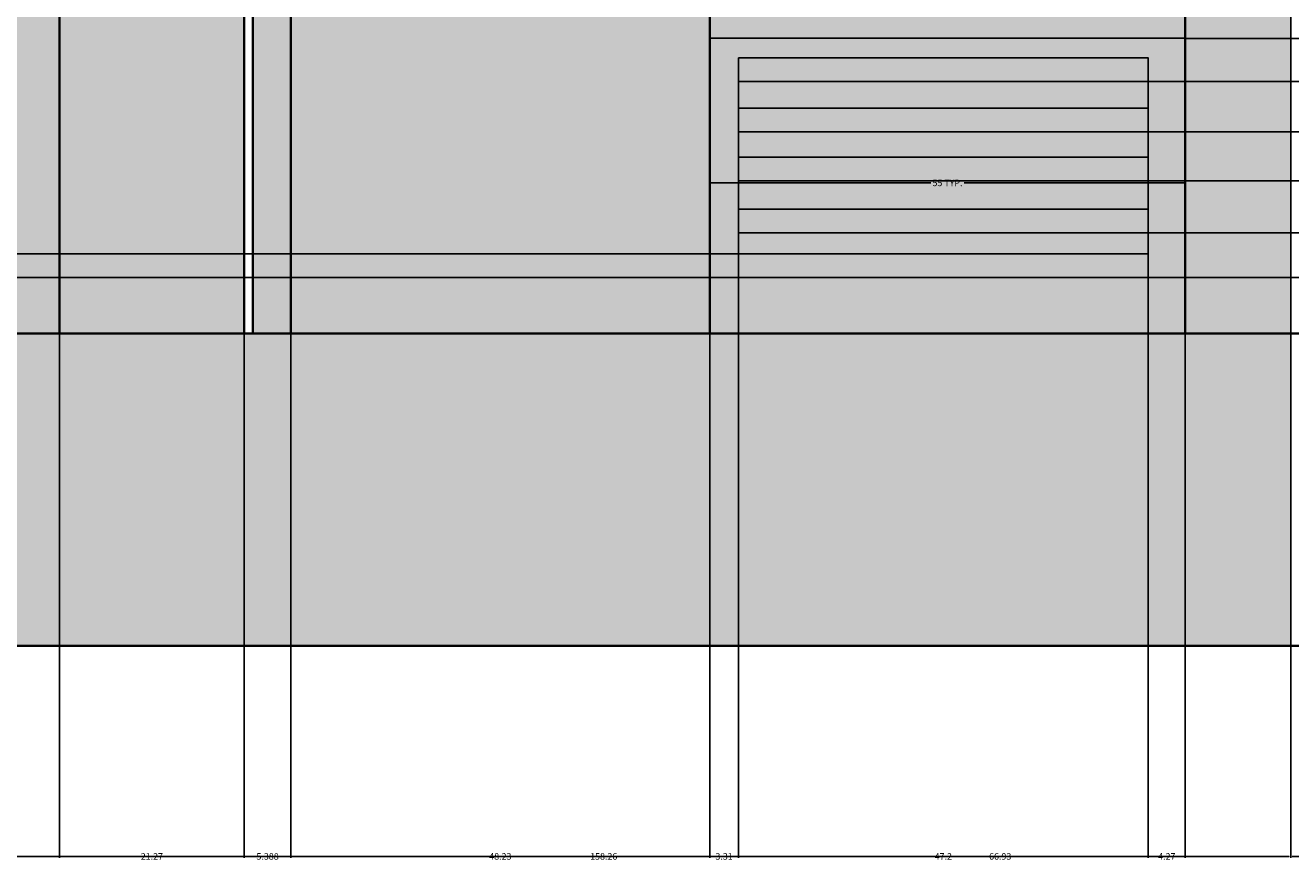
# Model space of a CAD drawing. Units: inches. Extents: x 62 to 566, y 66 to 528.
# Tile 3 of 20: x 138 to 284, y 66 to 162. Entities that reach past the tile are written whole.
import ezdxf

# ---------------------------------------------------------------- set-up
doc = ezdxf.new("R2010")
doc.units = ezdxf.units.IN
doc.header["$MEASUREMENT"] = 0
for name, color, linetype, lineweight in [('A-ANNO-DIMS', 2, 'Continuous', 18), ('A-ELEV', 7, 'Continuous', 35), ('A-GLAZ', 3, 'Continuous', 25), ('A-WALL-PATT', 8, 'Continuous', 13)]:
    doc.layers.add(name, color=color, linetype=linetype, lineweight=lineweight)
doc.styles.get("Standard").update_dxf_attribs({"font": 'arial.ttf'})
doc.dimstyles.get("Standard").update_dxf_attribs({"dimtxt": 0.75, "dimasz": 0.18, "dimexe": 0.18, "dimexo": 0.0625, "dimgap": 0.09, "dimtad": 0, "dimtih": 1, "dimtoh": 1, "dimdec": 4, "dimzin": 0, "dimdsep": 46, "dimlunit": 4, "dimtxsty": 'Standard', "dimcen": 0.09, "dimadec": 0, "dimazin": 0, "dimtfac": 1, "dimtdec": 4, "dimtofl": 0, "dimtmove": 0, "dimatfit": 3, "dimfxl": 1, "dimtolj": 1, "dimtzin": 0, "dimarcsym": 0})

# ---------------------------------------------------------------- blocks, each defined once
blk = doc.blocks.new('WIN-FRENCH-GRID')
for p, q in [((26.39, 108.06), (26.39, 83.9)), ((28.39, 108.06), (28.39, 83.9)), ((26.39, 83.9), (3, 83.9)), ((51.78, 83.9), (28.39, 83.9)), ((26.39, 81.9), (3, 81.9)), ((26.39, 81.9), (26.39, 41.97)), ((51.78, 81.9), (28.39, 81.9)), ((28.39, 81.9), (28.39, 41.97)), ((26.39, 41.97), (3, 41.97)), ((51.78, 41.97), (28.39, 41.97)), ((26.39, 39.97), (3, 39.97)), ((26.39, 39.97), (26.39, 3)), ((51.78, 39.97), (28.39, 39.97)), ((28.39, 39.97), (28.39, 3))]:
    blk.add_line(p, q)
blk.add_lwpolyline([(0, 111.06), (54.78, 111.06), (54.78, 0), (0, 0)], close=True)
for points in [[(3, 83.9), (3, 108.06), (26.39, 108.06)], [(28.39, 108.06), (51.78, 108.06), (51.78, 83.9)], [(3, 41.97), (3, 81.9)], [(51.78, 81.9), (51.78, 41.97)], [(26.39, 3), (3, 3), (3, 39.97)], [(51.78, 39.97), (51.78, 3), (28.39, 3)]]:
    blk.add_lwpolyline(points)
blk = doc.blocks.new('*D5')
at = {"layer": 'A-ANNO-DIMS', "color": 0, "lineweight": -2, "transparency": 16777216}
for p, q in [((272.12, 271.41), (288.9, 271.41)), ((288.72, 271.23), (288.72, 216.36)), ((288.72, 160.53), (288.72, 215.41)), ((272.12, 160.35), (288.9, 160.35))]:
    blk.add_line(p, q, dxfattribs=at)
at = {"layer": 'A-ANNO-DIMS', "color": 0, "transparency": 16777216}
for points in [[(288.69, 271.23), (288.75, 271.23), (288.72, 271.41)], [(288.69, 160.53), (288.75, 160.53), (288.72, 160.35)]]:
    blk.add_solid(points, dxfattribs=at)
at = {"layer": 'Defpoints', "color": 0, "transparency": 16777216}
for p in [(272.06, 271.41), (288.72, 271.41), (272.06, 160.35)]:
    blk.add_point(p, dxfattribs=at)
at = {"layer": 'A-ANNO-DIMS', "color": 0, "transparency": 16777216, "insert": (288.72, 215.88), "char_height": 0.75, "attachment_point": 5}
blk.add_mtext('\\A1;FRENCH WINDOW 111 TYP.', dxfattribs=at)
blk = doc.blocks.new('*D6')
at = {"layer": 'A-ANNO-DIMS', "color": 0, "lineweight": -2, "transparency": 16777216}
for p, q in [((217.28, 160.29), (217.28, 143.52)), ((272.06, 160.29), (272.06, 143.52)), ((217.46, 143.7), (242.75, 143.7)), ((271.88, 143.7), (246.58, 143.7))]:
    blk.add_line(p, q, dxfattribs=at)
at = {"layer": 'A-ANNO-DIMS', "color": 0, "transparency": 16777216}
for points in [[(217.46, 143.73), (217.46, 143.67), (217.28, 143.7)], [(271.88, 143.73), (271.88, 143.67), (272.06, 143.7)]]:
    blk.add_solid(points, dxfattribs=at)
at = {"layer": 'Defpoints', "color": 0, "transparency": 16777216}
for p in [(217.28, 160.35), (272.06, 160.35), (272.06, 143.7)]:
    blk.add_point(p, dxfattribs=at)
at = {"layer": 'A-ANNO-DIMS', "color": 0, "transparency": 16777216, "insert": (244.67, 143.7), "char_height": 0.75, "attachment_point": 5}
blk.add_mtext('\\A1;55 TYP.', dxfattribs=at)
blk = doc.blocks.new('*D8')
at = {"layer": 'A-ANNO-DIMS', "color": 0, "lineweight": -2, "transparency": 16777216}
for p, q in [((284.2, 271.35), (284.2, 65.94)), ((125.94, 126.31), (125.94, 65.94)), ((126.12, 66.12), (203.46, 66.12)), ((284.02, 66.12), (206.68, 66.12))]:
    blk.add_line(p, q, dxfattribs=at)
at = {"layer": 'A-ANNO-DIMS', "color": 0, "transparency": 16777216}
for points in [[(126.12, 66.15), (126.12, 66.09), (125.94, 66.12)], [(284.02, 66.15), (284.02, 66.09), (284.2, 66.12)]]:
    blk.add_solid(points, dxfattribs=at)
at = {"layer": 'Defpoints', "color": 0, "transparency": 16777216}
for p in [(284.2, 271.41), (125.94, 126.37), (284.2, 66.12)]:
    blk.add_point(p, dxfattribs=at)
at = {"layer": 'A-ANNO-DIMS', "color": 0, "transparency": 16777216, "insert": (205.07, 66.12), "char_height": 0.75, "attachment_point": 5}
blk.add_mtext('\\A1;158.26', dxfattribs=at)
blk = doc.blocks.new('*D9')
at = {"layer": 'A-ANNO-DIMS', "color": 0, "lineweight": -2, "transparency": 16777216}
for p, q in [((284.2, 271.35), (284.2, 65.94)), ((316.21, 126.31), (316.21, 65.94)), ((284.38, 66.12), (298.92, 66.12)), ((316.03, 66.12), (301.49, 66.12))]:
    blk.add_line(p, q, dxfattribs=at)
at = {"layer": 'A-ANNO-DIMS', "color": 0, "transparency": 16777216}
for points in [[(284.38, 66.15), (284.38, 66.09), (284.2, 66.12)], [(316.03, 66.15), (316.03, 66.09), (316.21, 66.12)]]:
    blk.add_solid(points, dxfattribs=at)
at = {"layer": 'Defpoints', "color": 0, "transparency": 16777216}
for p in [(284.2, 271.41), (316.21, 126.37), (316.21, 66.12)]:
    blk.add_point(p, dxfattribs=at)
at = {"layer": 'A-ANNO-DIMS', "color": 0, "transparency": 16777216, "insert": (300.21, 66.12), "char_height": 0.75, "attachment_point": 5}
blk.add_mtext('\\A1;32.01', dxfattribs=at)
blk = doc.blocks.new('*D16')
at = {"layer": 'A-ANNO-DIMS', "color": 0, "lineweight": -2, "transparency": 16777216}
for p, q in [((87.83, 126.37), (63.47, 126.37)), ((63.65, 126.19), (63.65, 108.84)), ((63.65, 90.55), (63.65, 107.9)), ((284.14, 90.37), (63.47, 90.37))]:
    blk.add_line(p, q, dxfattribs=at)
at = {"layer": 'A-ANNO-DIMS', "color": 0, "transparency": 16777216}
for points in [[(63.62, 126.19), (63.68, 126.19), (63.65, 126.37)], [(63.62, 90.55), (63.68, 90.55), (63.65, 90.37)]]:
    blk.add_solid(points, dxfattribs=at)
at = {"layer": 'Defpoints', "color": 0, "transparency": 16777216}
for p in [(63.65, 126.37), (87.9, 126.37), (284.2, 90.37)]:
    blk.add_point(p, dxfattribs=at)
at = {"layer": 'A-ANNO-DIMS', "color": 0, "transparency": 16777216, "insert": (63.65, 108.37), "char_height": 0.75, "attachment_point": 5}
blk.add_mtext('\\A1;36', dxfattribs=at)
blk = doc.blocks.new('*D35')
at = {"layer": 'A-ANNO-DIMS', "color": 0, "lineweight": -2, "transparency": 16777216}
for p, q in [((125.94, 461.98), (125.94, 65.94)), ((142.39, 445.04), (142.39, 65.94)), ((126.12, 66.12), (132.55, 66.12)), ((142.21, 66.12), (135.77, 66.12))]:
    blk.add_line(p, q, dxfattribs=at)
at = {"layer": 'A-ANNO-DIMS', "color": 0, "transparency": 16777216}
for points in [[(126.12, 66.15), (126.12, 66.09), (125.94, 66.12)], [(142.21, 66.15), (142.21, 66.09), (142.39, 66.12)]]:
    blk.add_solid(points, dxfattribs=at)
at = {"layer": 'Defpoints', "color": 0, "transparency": 16777216}
for p in [(125.94, 462.04), (142.39, 445.11), (142.39, 66.12)]:
    blk.add_point(p, dxfattribs=at)
at = {"layer": 'A-ANNO-DIMS', "color": 0, "transparency": 16777216, "insert": (134.16, 66.12), "char_height": 0.75, "attachment_point": 5}
blk.add_mtext('\\A1;16.443', dxfattribs=at)
blk = doc.blocks.new('*D36')
at = {"layer": 'A-ANNO-DIMS', "color": 0, "lineweight": -2, "transparency": 16777216}
for p, q in [((142.39, 445.04), (142.39, 65.94)), ((163.65, 427.41), (163.65, 65.94)), ((142.57, 66.12), (151.66, 66.12)), ((163.47, 66.12), (154.38, 66.12))]:
    blk.add_line(p, q, dxfattribs=at)
at = {"layer": 'A-ANNO-DIMS', "color": 0, "transparency": 16777216}
for points in [[(142.57, 66.15), (142.57, 66.09), (142.39, 66.12)], [(163.47, 66.15), (163.47, 66.09), (163.65, 66.12)]]:
    blk.add_solid(points, dxfattribs=at)
at = {"layer": 'Defpoints', "color": 0, "transparency": 16777216}
for p in [(142.39, 445.11), (163.65, 427.48), (163.65, 66.12)]:
    blk.add_point(p, dxfattribs=at)
at = {"layer": 'A-ANNO-DIMS', "color": 0, "transparency": 16777216, "insert": (153.02, 66.12), "char_height": 0.75, "attachment_point": 5}
blk.add_mtext('\\A1;21.27', dxfattribs=at)
blk = doc.blocks.new('*D37')
at = {"layer": 'A-ANNO-DIMS', "color": 0, "lineweight": -2, "transparency": 16777216}
for p, q in [((163.65, 427.41), (163.65, 65.94)), ((169.04, 420.53), (169.04, 65.94)), ((163.83, 66.12), (164.99, 66.12)), ((168.86, 66.12), (167.71, 66.12))]:
    blk.add_line(p, q, dxfattribs=at)
at = {"layer": 'A-ANNO-DIMS', "color": 0, "transparency": 16777216}
for points in [[(163.83, 66.15), (163.83, 66.09), (163.65, 66.12)], [(168.86, 66.15), (168.86, 66.09), (169.04, 66.12)]]:
    blk.add_solid(points, dxfattribs=at)
at = {"layer": 'Defpoints', "color": 0, "transparency": 16777216}
for p in [(163.65, 427.48), (169.04, 420.6), (169.04, 66.12)]:
    blk.add_point(p, dxfattribs=at)
at = {"layer": 'A-ANNO-DIMS', "color": 0, "transparency": 16777216, "insert": (166.35, 66.12), "char_height": 0.75, "attachment_point": 5}
blk.add_mtext('\\A1;5.388', dxfattribs=at)
blk = doc.blocks.new('*D38')
at = {"layer": 'A-ANNO-DIMS', "color": 0, "lineweight": -2, "transparency": 16777216}
for p, q in [((169.04, 420.53), (169.04, 65.94)), ((217.28, 420.53), (217.28, 65.94)), ((169.22, 66.12), (191.79, 66.12)), ((217.1, 66.12), (194.53, 66.12))]:
    blk.add_line(p, q, dxfattribs=at)
at = {"layer": 'A-ANNO-DIMS', "color": 0, "transparency": 16777216}
for points in [[(169.22, 66.15), (169.22, 66.09), (169.04, 66.12)], [(217.1, 66.15), (217.1, 66.09), (217.28, 66.12)]]:
    blk.add_solid(points, dxfattribs=at)
at = {"layer": 'Defpoints', "color": 0, "transparency": 16777216}
for p in [(169.04, 420.6), (217.28, 420.6), (217.28, 66.12)]:
    blk.add_point(p, dxfattribs=at)
at = {"layer": 'A-ANNO-DIMS', "color": 0, "transparency": 16777216, "insert": (193.16, 66.12), "char_height": 0.75, "attachment_point": 5}
blk.add_mtext('\\A1;48.23', dxfattribs=at)
blk = doc.blocks.new('*D39')
at = {"layer": 'A-ANNO-DIMS', "color": 0, "lineweight": -2, "transparency": 16777216}
for p, q in [((284.2, 445.04), (284.2, 65.94)), ((217.28, 420.53), (217.28, 65.94)), ((217.46, 66.12), (249.38, 66.12)), ((284.02, 66.12), (252.1, 66.12))]:
    blk.add_line(p, q, dxfattribs=at)
at = {"layer": 'A-ANNO-DIMS', "color": 0, "transparency": 16777216}
for points in [[(217.46, 66.15), (217.46, 66.09), (217.28, 66.12)], [(284.02, 66.15), (284.02, 66.09), (284.2, 66.12)]]:
    blk.add_solid(points, dxfattribs=at)
at = {"layer": 'Defpoints', "color": 0, "transparency": 16777216}
for p in [(284.2, 445.11), (217.28, 420.6), (284.2, 66.12)]:
    blk.add_point(p, dxfattribs=at)
at = {"layer": 'A-ANNO-DIMS', "color": 0, "transparency": 16777216, "insert": (250.74, 66.12), "char_height": 0.75, "attachment_point": 5}
blk.add_mtext('\\A1;66.93', dxfattribs=at)
blk = doc.blocks.new('*D40')
at = {"layer": 'A-ANNO-DIMS', "color": 0, "lineweight": -2, "transparency": 16777216}
for p, q in [((284.2, 445.04), (284.2, 65.94)), ((316.21, 417.64), (316.21, 65.94)), ((284.38, 66.12), (298.92, 66.12)), ((316.03, 66.12), (301.49, 66.12))]:
    blk.add_line(p, q, dxfattribs=at)
at = {"layer": 'A-ANNO-DIMS', "color": 0, "transparency": 16777216}
for points in [[(284.38, 66.15), (284.38, 66.09), (284.2, 66.12)], [(316.03, 66.15), (316.03, 66.09), (316.21, 66.12)]]:
    blk.add_solid(points, dxfattribs=at)
at = {"layer": 'Defpoints', "color": 0, "transparency": 16777216}
for p in [(284.2, 445.11), (316.21, 417.71), (316.21, 66.12)]:
    blk.add_point(p, dxfattribs=at)
at = {"layer": 'A-ANNO-DIMS', "color": 0, "transparency": 16777216, "insert": (300.21, 66.12), "char_height": 0.75, "attachment_point": 5}
blk.add_mtext('\\A1;32.01', dxfattribs=at)
blk = doc.blocks.new('*D57')
at = {"layer": 'A-ANNO-DIMS', "color": 0, "lineweight": -2, "transparency": 16777216}
for p, q in [((316.21, 126.31), (316.21, 65.94)), ((284.2, 90.31), (284.2, 65.94)), ((284.38, 66.12), (298.92, 66.12)), ((316.03, 66.12), (301.49, 66.12))]:
    blk.add_line(p, q, dxfattribs=at)
at = {"layer": 'A-ANNO-DIMS', "color": 0, "transparency": 16777216}
for points in [[(284.38, 66.15), (284.38, 66.09), (284.2, 66.12)], [(316.03, 66.15), (316.03, 66.09), (316.21, 66.12)]]:
    blk.add_solid(points, dxfattribs=at)
at = {"layer": 'Defpoints', "color": 0, "transparency": 16777216}
for p in [(316.21, 126.37), (284.2, 90.37), (316.21, 66.12)]:
    blk.add_point(p, dxfattribs=at)
at = {"layer": 'A-ANNO-DIMS', "color": 0, "transparency": 16777216, "insert": (300.21, 66.12), "char_height": 0.75, "attachment_point": 5}
blk.add_mtext('\\A1;32.01', dxfattribs=at)
blk = doc.blocks.new('*D73')
at = {"layer": 'A-ANNO-DIMS', "color": 0, "lineweight": -2, "transparency": 16777216}
for p, q in [((316.15, 236.66), (63.47, 236.66)), ((63.65, 236.48), (63.65, 181.99)), ((63.65, 126.55), (63.65, 181.04)), ((316.15, 126.37), (63.47, 126.37))]:
    blk.add_line(p, q, dxfattribs=at)
at = {"layer": 'A-ANNO-DIMS', "color": 0, "transparency": 16777216}
for points in [[(63.62, 236.48), (63.68, 236.48), (63.65, 236.66)], [(63.62, 126.55), (63.68, 126.55), (63.65, 126.37)]]:
    blk.add_solid(points, dxfattribs=at)
at = {"layer": 'Defpoints', "color": 0, "transparency": 16777216}
for p in [(63.65, 236.66), (316.21, 236.66), (316.21, 126.37)]:
    blk.add_point(p, dxfattribs=at)
at = {"layer": 'A-ANNO-DIMS', "color": 0, "transparency": 16777216, "insert": (63.65, 181.52), "char_height": 0.75, "attachment_point": 5}
blk.add_mtext('\\A1;110.3', dxfattribs=at)
blk = doc.blocks.new('*D82')
at = {"layer": 'A-ANNO-DIMS', "color": 0, "lineweight": -2, "transparency": 16777216}
for p, q in [((296.38, 279.98), (296.38, 65.94)), ((284.2, 271.35), (284.2, 65.94)), ((284.38, 66.12), (288.68, 66.12)), ((296.2, 66.12), (291.9, 66.12))]:
    blk.add_line(p, q, dxfattribs=at)
at = {"layer": 'A-ANNO-DIMS', "color": 0, "transparency": 16777216}
for points in [[(284.38, 66.15), (284.38, 66.09), (284.2, 66.12)], [(296.2, 66.15), (296.2, 66.09), (296.38, 66.12)]]:
    blk.add_solid(points, dxfattribs=at)
at = {"layer": 'Defpoints', "color": 0, "transparency": 16777216}
for p in [(296.38, 280.04), (284.2, 271.41), (296.38, 66.12)]:
    blk.add_point(p, dxfattribs=at)
at = {"layer": 'A-ANNO-DIMS', "color": 0, "transparency": 16777216, "insert": (290.29, 66.12), "char_height": 0.75, "attachment_point": 5}
blk.add_mtext('\\A1;12.173', dxfattribs=at)
blk = doc.blocks.new('*D113')
at = {"layer": 'A-ANNO-DIMS', "color": 0, "lineweight": -2, "transparency": 16777216}
for p, q in [((217.28, 160.29), (217.28, 65.94)), ((220.59, 158.04), (220.59, 65.94)), ((217.46, 66.12), (217.94, 66.12)), ((220.41, 66.12), (219.92, 66.12))]:
    blk.add_line(p, q, dxfattribs=at)
at = {"layer": 'A-ANNO-DIMS', "color": 0, "transparency": 16777216}
for points in [[(217.46, 66.15), (217.46, 66.09), (217.28, 66.12)], [(220.41, 66.15), (220.41, 66.09), (220.59, 66.12)]]:
    blk.add_solid(points, dxfattribs=at)
at = {"layer": 'Defpoints', "color": 0, "transparency": 16777216}
for p in [(217.28, 160.35), (220.59, 158.1), (220.59, 66.12)]:
    blk.add_point(p, dxfattribs=at)
at = {"layer": 'A-ANNO-DIMS', "color": 0, "transparency": 16777216, "insert": (218.93, 66.12), "char_height": 0.75, "attachment_point": 5}
blk.add_mtext('\\A1;3.31', dxfattribs=at)
blk = doc.blocks.new('*D114')
at = {"layer": 'A-ANNO-DIMS', "color": 0, "lineweight": -2, "transparency": 16777216}
for p, q in [((220.59, 158.04), (220.59, 65.94)), ((267.79, 158.04), (267.79, 65.94)), ((220.77, 66.12), (243.12, 66.12)), ((267.61, 66.12), (245.27, 66.12))]:
    blk.add_line(p, q, dxfattribs=at)
at = {"layer": 'A-ANNO-DIMS', "color": 0, "transparency": 16777216}
for points in [[(220.77, 66.15), (220.77, 66.09), (220.59, 66.12)], [(267.61, 66.15), (267.61, 66.09), (267.79, 66.12)]]:
    blk.add_solid(points, dxfattribs=at)
at = {"layer": 'Defpoints', "color": 0, "transparency": 16777216}
for p in [(220.59, 158.1), (267.79, 158.1), (267.79, 66.12)]:
    blk.add_point(p, dxfattribs=at)
at = {"layer": 'A-ANNO-DIMS', "color": 0, "transparency": 16777216, "insert": (244.19, 66.12), "char_height": 0.75, "attachment_point": 5}
blk.add_mtext('\\A1;47.2', dxfattribs=at)
blk = doc.blocks.new('*D115')
at = {"layer": 'A-ANNO-DIMS', "color": 0, "lineweight": -2, "transparency": 16777216}
for p, q in [((272.06, 160.29), (272.06, 65.94)), ((267.79, 158.04), (267.79, 65.94)), ((267.97, 66.12), (268.85, 66.12)), ((271.88, 66.12), (271, 66.12))]:
    blk.add_line(p, q, dxfattribs=at)
at = {"layer": 'A-ANNO-DIMS', "color": 0, "transparency": 16777216}
for points in [[(267.97, 66.15), (267.97, 66.09), (267.79, 66.12)], [(271.88, 66.15), (271.88, 66.09), (272.06, 66.12)]]:
    blk.add_solid(points, dxfattribs=at)
at = {"layer": 'Defpoints', "color": 0, "transparency": 16777216}
for p in [(272.06, 160.35), (267.79, 158.1), (272.06, 66.12)]:
    blk.add_point(p, dxfattribs=at)
at = {"layer": 'A-ANNO-DIMS', "color": 0, "transparency": 16777216, "insert": (269.93, 66.12), "char_height": 0.75, "attachment_point": 5}
blk.add_mtext('\\A1;4.27', dxfattribs=at)
blk = doc.blocks.new('*D116')
at = {"layer": 'A-ANNO-DIMS', "color": 0, "lineweight": -2, "transparency": 16777216}
for p, q in [((267.86, 132.79), (564.47, 132.79)), ((564.29, 132.61), (564.29, 130.05)), ((564.29, 126.55), (564.29, 129.11)), ((272.12, 126.37), (564.47, 126.37))]:
    blk.add_line(p, q, dxfattribs=at)
at = {"layer": 'A-ANNO-DIMS', "color": 0, "transparency": 16777216}
for points in [[(564.26, 132.61), (564.32, 132.61), (564.29, 132.79)], [(564.26, 126.55), (564.32, 126.55), (564.29, 126.37)]]:
    blk.add_solid(points, dxfattribs=at)
at = {"layer": 'Defpoints', "color": 0, "transparency": 16777216}
for p in [(267.79, 132.79), (564.29, 132.79), (272.06, 126.37)]:
    blk.add_point(p, dxfattribs=at)
at = {"layer": 'A-ANNO-DIMS', "color": 0, "transparency": 16777216, "insert": (564.29, 129.58), "char_height": 0.75, "attachment_point": 5}
blk.add_mtext('\\A1;6.426', dxfattribs=at)
blk = doc.blocks.new('*D117')
at = {"layer": 'A-ANNO-DIMS', "color": 0, "lineweight": -2, "transparency": 16777216}
for p, q in [((267.86, 137.96), (564.47, 137.96)), ((564.29, 137.78), (564.29, 135.85)), ((564.29, 132.97), (564.29, 134.91)), ((267.86, 132.79), (564.47, 132.79))]:
    blk.add_line(p, q, dxfattribs=at)
at = {"layer": 'A-ANNO-DIMS', "color": 0, "transparency": 16777216}
for points in [[(564.26, 137.78), (564.32, 137.78), (564.29, 137.96)], [(564.26, 132.97), (564.32, 132.97), (564.29, 132.79)]]:
    blk.add_solid(points, dxfattribs=at)
at = {"layer": 'Defpoints', "color": 0, "transparency": 16777216}
for p in [(267.79, 137.96), (564.29, 137.96), (267.79, 132.79)]:
    blk.add_point(p, dxfattribs=at)
at = {"layer": 'A-ANNO-DIMS', "color": 0, "transparency": 16777216, "insert": (564.29, 135.38), "char_height": 0.75, "attachment_point": 5}
blk.add_mtext('\\A1;5.17', dxfattribs=at)
blk = doc.blocks.new('*D118')
at = {"layer": 'A-ANNO-DIMS', "color": 0, "lineweight": -2, "transparency": 16777216}
for p, q in [((267.86, 143.95), (564.47, 143.95)), ((564.29, 143.77), (564.29, 141.43)), ((564.29, 138.14), (564.29, 140.49)), ((267.86, 137.96), (564.47, 137.96))]:
    blk.add_line(p, q, dxfattribs=at)
at = {"layer": 'A-ANNO-DIMS', "color": 0, "transparency": 16777216}
for points in [[(564.26, 143.77), (564.32, 143.77), (564.29, 143.95)], [(564.26, 138.14), (564.32, 138.14), (564.29, 137.96)]]:
    blk.add_solid(points, dxfattribs=at)
at = {"layer": 'Defpoints', "color": 0, "transparency": 16777216}
for p in [(267.79, 143.95), (564.29, 143.95), (267.79, 137.96)]:
    blk.add_point(p, dxfattribs=at)
at = {"layer": 'A-ANNO-DIMS', "color": 0, "transparency": 16777216, "insert": (564.29, 140.96), "char_height": 0.75, "attachment_point": 5}
blk.add_mtext('\\A1;5.986', dxfattribs=at)
blk = doc.blocks.new('*D119')
at = {"layer": 'A-ANNO-DIMS', "color": 0, "lineweight": -2, "transparency": 16777216}
for p, q in [((267.86, 149.57), (564.47, 149.57)), ((564.29, 149.39), (564.29, 147.24)), ((564.29, 144.13), (564.29, 146.29)), ((267.86, 143.95), (564.47, 143.95))]:
    blk.add_line(p, q, dxfattribs=at)
at = {"layer": 'A-ANNO-DIMS', "color": 0, "transparency": 16777216}
for points in [[(564.26, 149.39), (564.32, 149.39), (564.29, 149.57)], [(564.26, 144.13), (564.32, 144.13), (564.29, 143.95)]]:
    blk.add_solid(points, dxfattribs=at)
at = {"layer": 'Defpoints', "color": 0, "transparency": 16777216}
for p in [(267.79, 149.57), (564.29, 149.57), (267.79, 143.95)]:
    blk.add_point(p, dxfattribs=at)
at = {"layer": 'A-ANNO-DIMS', "color": 0, "transparency": 16777216, "insert": (564.29, 146.76), "char_height": 0.75, "attachment_point": 5}
blk.add_mtext('\\A1;5.624', dxfattribs=at)
blk = doc.blocks.new('*D120')
at = {"layer": 'A-ANNO-DIMS', "color": 0, "lineweight": -2, "transparency": 16777216}
for p, q in [((267.86, 155.38), (564.47, 155.38)), ((564.29, 155.2), (564.29, 152.95)), ((564.29, 149.75), (564.29, 152)), ((267.86, 149.57), (564.47, 149.57))]:
    blk.add_line(p, q, dxfattribs=at)
at = {"layer": 'A-ANNO-DIMS', "color": 0, "transparency": 16777216}
for points in [[(564.26, 155.2), (564.32, 155.2), (564.29, 155.38)], [(564.26, 149.75), (564.32, 149.75), (564.29, 149.57)]]:
    blk.add_solid(points, dxfattribs=at)
at = {"layer": 'Defpoints', "color": 0, "transparency": 16777216}
for p in [(267.79, 155.38), (564.29, 155.38), (267.79, 149.57)]:
    blk.add_point(p, dxfattribs=at)
at = {"layer": 'A-ANNO-DIMS', "color": 0, "transparency": 16777216, "insert": (564.29, 152.48), "char_height": 0.75, "attachment_point": 5}
blk.add_mtext('\\A1;5.805', dxfattribs=at)
blk = doc.blocks.new('*D121')
at = {"layer": 'A-ANNO-DIMS', "color": 0, "lineweight": -2, "transparency": 16777216}
for p, q in [((272.12, 160.35), (564.47, 160.35)), ((564.29, 160.17), (564.29, 158.34)), ((564.29, 155.56), (564.29, 157.39)), ((267.86, 155.38), (564.47, 155.38))]:
    blk.add_line(p, q, dxfattribs=at)
at = {"layer": 'A-ANNO-DIMS', "color": 0, "transparency": 16777216}
for points in [[(564.26, 160.17), (564.32, 160.17), (564.29, 160.35)], [(564.26, 155.56), (564.32, 155.56), (564.29, 155.38)]]:
    blk.add_solid(points, dxfattribs=at)
at = {"layer": 'Defpoints', "color": 0, "transparency": 16777216}
for p in [(272.06, 160.35), (564.29, 160.35), (267.79, 155.38)]:
    blk.add_point(p, dxfattribs=at)
at = {"layer": 'A-ANNO-DIMS', "color": 0, "transparency": 16777216, "insert": (564.29, 157.87), "char_height": 0.75, "attachment_point": 5}
blk.add_mtext('\\A1;4.975', dxfattribs=at)
blk = doc.blocks.new('*D122')
at = {"layer": 'A-ANNO-DIMS', "color": 0, "lineweight": -2, "transparency": 16777216}
for p, q in [((269.12, 163.35), (564.47, 163.35)), ((564.29, 163.17), (564.29, 162.33)), ((272.12, 160.35), (564.47, 160.35)), ((564.29, 160.53), (564.29, 161.38))]:
    blk.add_line(p, q, dxfattribs=at)
at = {"layer": 'A-ANNO-DIMS', "color": 0, "transparency": 16777216}
for points in [[(564.26, 163.17), (564.32, 163.17), (564.29, 163.35)], [(564.26, 160.53), (564.32, 160.53), (564.29, 160.35)]]:
    blk.add_solid(points, dxfattribs=at)
at = {"layer": 'Defpoints', "color": 0, "transparency": 16777216}
for p in [(269.06, 163.35), (564.29, 163.35), (272.06, 160.35)]:
    blk.add_point(p, dxfattribs=at)
at = {"layer": 'A-ANNO-DIMS', "color": 0, "transparency": 16777216, "insert": (564.29, 161.85), "char_height": 0.75, "attachment_point": 5}
blk.add_mtext('\\A1;3', dxfattribs=at)
blk = doc.blocks.new('*D129')
at = {"layer": 'A-ANNO-DIMS', "color": 0, "lineweight": -2, "transparency": 16777216}
for p, q in [((220.53, 135.52), (63.47, 135.52)), ((63.65, 135.34), (63.65, 134.62)), ((220.53, 132.79), (63.47, 132.79)), ((63.65, 132.97), (63.65, 133.69))]:
    blk.add_line(p, q, dxfattribs=at)
at = {"layer": 'A-ANNO-DIMS', "color": 0, "transparency": 16777216}
for points in [[(63.62, 135.34), (63.68, 135.34), (63.65, 135.52)], [(63.62, 132.97), (63.68, 132.97), (63.65, 132.79)]]:
    blk.add_solid(points, dxfattribs=at)
at = {"layer": 'Defpoints', "color": 0, "transparency": 16777216}
for p in [(63.65, 135.52), (220.59, 135.52), (220.59, 132.79)]:
    blk.add_point(p, dxfattribs=at)
at = {"layer": 'A-ANNO-DIMS', "color": 0, "transparency": 16777216, "insert": (63.65, 134.16), "char_height": 0.75, "attachment_point": 5}
blk.add_mtext('\\A1;2.721', dxfattribs=at)

msp = doc.modelspace()

# ---------------------------------------------------------------- hatches: boundary and pattern name
at = {"layer": 'A-WALL-PATT'}
h = msp.add_hatch(color=256, dxfattribs=at)
h.dxf.hatch_style = 1
h.paths.add_polyline_path([(416.0836, 462.0423), (125.9418, 462.0423), (125.9418, 414.3686), (125.9418, 270.3686), (125.9418, 126.3686), (142.3851, 126.3686), (142.3851, 270.3686), (142.3851, 414.3686), (142.3851, 445.1064), (284.2021, 445.1064), (416.0836, 445.1064)])
h.paths.add_polyline_path([(435.3945, 503.0423), (426.3652, 503.0423), (120.4058, 503.0423), (120.4058, 501.0423), (125.9418, 501.0423), (416.0836, 501.0423), (426.3652, 501.0423), (430.6938, 501.0423), (435.3945, 501.0423)])
h.paths.add_polyline_path([(439.6878, 352.4848), (392.4793, 352.4848), (392.4793, 307.4128), (217.2752, 307.4128), (217.2752, 295.4098), (217.2752, 271.4128), (272.0586, 271.4128), (439.6878, 271.4128)])
h.paths.add_polyline_path([(248.0143, 297.1682), (255.6783, 297.1682), (255.6783, 280.0423), (248.0143, 280.0423)], flags=16)
h.paths.add_polyline_path([(235.4641, 280.0423), (227.8001, 280.0423), (227.8001, 297.1682), (235.4641, 297.1682)], flags=16)
h.paths.add_polyline_path([(270.4427, 297.1682), (278.1067, 297.1682), (278.1067, 280.0423), (270.4427, 280.0423)], flags=16)
h.paths.add_polyline_path([(296.3755, 297.1682), (304.0395, 297.1682), (304.0395, 280.0423), (296.3755, 280.0423)], flags=16)
h.paths.add_polyline_path([(319.2543, 297.1682), (326.9183, 297.1682), (326.9183, 280.0423), (319.2543, 280.0423)], flags=16)
h.paths.add_polyline_path([(341.2622, 297.1682), (348.9262, 297.1682), (348.9262, 280.0423), (341.2622, 280.0423)], flags=16)
h.paths.add_polyline_path([(389.2857, 298.3985), (433.8102, 298.3985), (433.8102, 294.9497), (389.2857, 294.9497)], flags=16)
h.paths.add_polyline_path([(389.2857, 291.6038), (433.8102, 291.6038), (433.8102, 288.155), (389.2857, 288.155)], flags=16)
h.paths.add_polyline_path([(389.2857, 284.9607), (433.8102, 284.9607), (433.8102, 281.5119), (389.2857, 281.5119)], flags=16)
h.paths.add_polyline_path([(403.5849, 311.4736), (403.5849, 317.4388), (433.1636, 317.4388), (433.1636, 311.4736)], flags=16)
h.paths.add_polyline_path([(403.5849, 323.1329), (403.5849, 329.0982), (433.1636, 329.0982), (433.1636, 323.1329)], flags=16)
h.paths.add_polyline_path([(403.5849, 334.5211), (403.5849, 340.4863), (433.1636, 340.4863), (433.1636, 334.5211)], flags=16)
h.paths.add_polyline_path([(272.0586, 160.3545), (217.2752, 160.3545), (217.2752, 129.0504), (217.2752, 126.3686), (272.0586, 126.3686)], flags=17)
h.paths.add_polyline_path([(220.5897, 149.5749), (220.5897, 152.296), (267.7931, 152.296), (267.7931, 149.5749)], flags=16)
h.paths.add_polyline_path([(267.7931, 146.6724), (267.7931, 143.9513), (220.5897, 143.9513), (220.5897, 146.6724)], flags=16)
h.paths.add_polyline_path([(220.5897, 155.3799), (220.5897, 158.101), (267.7931, 158.101), (267.7931, 155.3799)], flags=16)
h.paths.add_polyline_path([(267.7931, 140.686), (267.7931, 137.9649), (220.5897, 137.9649), (220.5897, 140.686)], flags=16)
h.paths.add_polyline_path([(267.7931, 135.516), (267.7931, 132.7949), (220.5897, 132.7949), (220.5897, 135.516)], flags=16)
h = msp.add_hatch(dxfattribs=at)
h.set_pattern_fill('ANSI36', color=256, scale=8.8)
h.paths.add_polyline_path([(217.2752, 420.597), (169.0431, 420.597), (169.0431, 126.3686), (217.2752, 126.3686), (217.2752, 129.0504), (217.2752, 271.4128), (217.2752, 295.4128), (217.2752, 307.4128)])
h.paths.add_polyline_path([(282.3509, 501.0423), (125.9418, 501.0423), (125.9418, 465.0423), (282.3509, 465.0423)])
h.paths.add_polyline_path([(209.709, 476.6506), (202.045, 476.6506), (202.045, 493.7764), (209.709, 493.7764)], flags=16)
h.paths.add_polyline_path([(193.9913, 476.6506), (186.3273, 476.6506), (186.3273, 493.7764), (193.9913, 493.7764)], flags=16)
h.paths.add_polyline_path([(177.9243, 476.6506), (170.2603, 476.6506), (170.2603, 493.7764), (177.9243, 493.7764)], flags=16)
h.paths.add_polyline_path([(163.2545, 476.3015), (155.5905, 476.3015), (155.5905, 493.4274), (163.2545, 493.4274)], flags=16)
h.paths.add_polyline_path([(148.2354, 476.3015), (140.5713, 476.3015), (140.5713, 493.4274), (148.2354, 493.4274)], flags=16)
h.paths.add_polyline_path([(284.2021, 126.3686), (87.8962, 126.3686), (87.8962, 114.3686), (87.8962, 90.3686), (284.2021, 90.3686)])
h.paths.add_polyline_path([(474.1214, 126.3686), (396.433, 126.3686), (396.433, 90.3686), (474.1214, 90.3686)])
h = msp.add_hatch(color=256, dxfattribs=at)
h.dxf.hatch_style = 1
h.paths.add_polyline_path([(416.0836, 501.0423), (282.3509, 501.0423), (282.3509, 465.0423), (416.0836, 465.0423)])
h.paths.add_polyline_path([(284.2021, 420.597), (272.0586, 420.597), (272.0586, 309.5388), (272.0586, 307.4128), (284.2021, 307.4128)], flags=17)
h.paths.add_polyline_path([(284.2021, 445.1064), (142.3851, 445.1064), (142.3851, 414.3686), (142.3851, 270.3686), (142.3851, 126.3686), (163.6548, 126.3686), (163.6548, 270.5016), (163.6548, 414.5016), (163.6548, 427.4752), (284.2021, 427.4752)])
h.paths.add_polyline_path([(235.4641, 297.1682), (227.8001, 297.1682), (227.8001, 280.0423), (235.4641, 280.0423)], flags=17)
h.paths.add_polyline_path([(255.6783, 297.1682), (248.0143, 297.1682), (248.0143, 280.0423), (255.6783, 280.0423)], flags=17)
h.paths.add_polyline_path([(278.1067, 297.1682), (270.4427, 297.1682), (270.4427, 280.0423), (278.1067, 280.0423)], flags=17)
h.paths.add_polyline_path([(304.0395, 297.1682), (296.3755, 297.1682), (296.3755, 280.0423), (304.0395, 280.0423)])
h.paths.add_polyline_path([(326.9183, 297.1682), (319.2543, 297.1682), (319.2543, 280.0423), (326.9183, 280.0423)])
h.paths.add_polyline_path([(348.9262, 297.1682), (341.2622, 297.1682), (341.2622, 280.0423), (348.9262, 280.0423)])
h.paths.add_polyline_path([(433.8102, 284.9607), (389.2857, 284.9607), (389.2857, 281.5119), (433.8102, 281.5119)])
h.paths.add_polyline_path([(433.8102, 291.6038), (389.2857, 291.6038), (389.2857, 288.155), (433.8102, 288.155)])
h.paths.add_polyline_path([(433.8102, 298.3985), (389.2857, 298.3985), (389.2857, 294.9497), (433.8102, 294.9497)])
h.paths.add_polyline_path([(433.1636, 317.4388), (403.5849, 317.4388), (403.5849, 311.4736), (433.1636, 311.4736)])
h.paths.add_polyline_path([(433.1636, 329.0982), (403.5849, 329.0982), (403.5849, 323.1329), (433.1636, 323.1329)])
h.paths.add_polyline_path([(433.1636, 340.4863), (403.5849, 340.4863), (403.5849, 334.5211), (433.1636, 334.5211)])
h.paths.add_polyline_path([(284.2021, 271.4128), (272.0586, 271.4128), (272.0586, 160.3545), (272.0586, 126.3686), (284.2021, 126.3686)])
h.paths.add_polyline_path([(267.7931, 158.101), (220.5897, 158.101), (220.5897, 155.3799), (267.7931, 155.3799)], flags=17)
h.paths.add_polyline_path([(267.7931, 152.296), (220.5897, 152.296), (220.5897, 149.5749), (267.7931, 149.5749)], flags=17)
h.paths.add_polyline_path([(267.7931, 146.6724), (220.5897, 146.6724), (220.5897, 143.9513), (267.7931, 143.9513)], flags=17)
h.paths.add_polyline_path([(267.7931, 140.686), (220.5897, 140.686), (220.5897, 137.9649), (267.7931, 137.9649)], flags=17)
h.paths.add_polyline_path([(267.7931, 135.516), (220.5897, 135.516), (220.5897, 132.7949), (267.7931, 132.7949)], flags=17)
h.paths.add_polyline_path([(148.2354, 493.4274), (140.5713, 493.4274), (140.5713, 476.3015), (148.2354, 476.3015)])
h.paths.add_polyline_path([(163.2545, 493.4274), (155.5905, 493.4274), (155.5905, 476.3015), (163.2545, 476.3015)])
h.paths.add_polyline_path([(177.9243, 493.7764), (170.2603, 493.7764), (170.2603, 476.6506), (177.9243, 476.6506)])
h.paths.add_polyline_path([(193.9913, 493.7764), (186.3273, 493.7764), (186.3273, 476.6506), (193.9913, 476.6506)])
h.paths.add_polyline_path([(209.709, 493.7764), (202.045, 493.7764), (202.045, 476.6506), (209.709, 476.6506)])
h = msp.add_hatch(color=256, dxfattribs=at)
h.dxf.hatch_style = 1
h.paths.add_polyline_path([(430.6938, 462.0423), (416.0836, 462.0423), (416.0836, 445.1064), (430.6938, 445.1064)])
h.paths.add_polyline_path([(169.0431, 420.597), (284.2021, 420.597), (284.2021, 426.4752), (164.6548, 426.4752), (164.6548, 414.5016), (164.6548, 126.3686), (169.0431, 126.3686)])
h = msp.add_hatch(color=256, dxfattribs=at)
h.dxf.hatch_style = 1
h.paths.add_polyline_path([(272.0586, 420.597), (217.2752, 420.597), (217.2752, 309.5388), (272.0586, 309.5388)])
h.paths.add_polyline_path([(245.6669, 393.435), (245.6669, 417.597), (269.0586, 417.597), (269.0586, 393.435)], flags=16)
h.paths.add_polyline_path([(245.6669, 391.435), (269.0586, 391.435), (269.0586, 351.5079), (245.6669, 351.5079)], flags=16)
h.paths.add_polyline_path([(243.6669, 393.435), (220.2752, 393.435), (220.2752, 417.597), (243.6669, 417.597)], flags=16)
h.paths.add_polyline_path([(243.6669, 391.435), (243.6669, 351.5079), (220.2752, 351.5079), (220.2752, 391.435)], flags=16)
h.paths.add_polyline_path([(245.6669, 349.5079), (269.0586, 349.5079), (269.0586, 312.5388), (245.6669, 312.5388)], flags=16)
h.paths.add_polyline_path([(243.6669, 349.5079), (243.6669, 312.5388), (220.2752, 312.5388), (220.2752, 349.5079)], flags=16)
h.paths.add_polyline_path([(272.0586, 271.4128), (217.2752, 271.4128), (217.2752, 160.3545), (272.0586, 160.3545)])
h.paths.add_polyline_path([(243.6669, 268.4128), (243.6669, 244.2507), (220.2752, 244.2507), (220.2752, 268.4128)], flags=16)
h.paths.add_polyline_path([(245.6669, 268.4128), (269.0586, 268.4128), (269.0586, 244.2507), (245.6669, 244.2507)], flags=16)
h.paths.add_polyline_path([(243.6669, 242.2507), (243.6669, 202.3236), (220.2752, 202.3236), (220.2752, 242.2507)], flags=16)
h.paths.add_polyline_path([(245.6669, 242.2507), (269.0586, 242.2507), (269.0586, 202.3236), (245.6669, 202.3236)], flags=16)
h.paths.add_polyline_path([(243.6669, 200.3236), (243.6669, 163.3545), (220.2752, 163.3545), (220.2752, 200.3236)], flags=16)
h.paths.add_polyline_path([(245.6669, 200.3236), (269.0586, 200.3236), (269.0586, 163.3545), (245.6669, 163.3545)], flags=16)
h.paths.add_polyline_path([(272.0586, 309.5388), (217.2752, 309.5388), (217.2752, 307.4128), (272.0586, 307.4128)])

# ---------------------------------------------------------------- linework, layer by layer
at = {"layer": 'A-ELEV'}
for p, q in [((169.0431, 126.3686), (169.0431, 420.597)), ((217.2752, 129.0504), (217.2752, 271.4128)), ((272.0586, 126.3686), (272.0586, 271.4128)), ((142.3851, 126.3686), (142.3851, 270.3686)), ((217.2752, 129.0504), (217.2752, 126.3686)), ((87.8962, 126.3686), (396.433, 126.3686)), ((87.8962, 90.3686), (396.433, 90.3686))]:
    msp.add_line(p, q, dxfattribs=at)
for points in [[(163.6548, 126.3686), (163.6548, 414.5016), (163.6548, 427.4752), (284.2021, 427.4752)], [(164.6548, 126.3686), (164.6548, 414.5016), (164.6548, 426.4752), (284.2021, 426.4752)]]:
    msp.add_lwpolyline(points, dxfattribs=at)
at = {"layer": 'A-GLAZ'}
for points in [[(220.5897, 158.101), (267.7931, 158.101), (267.7931, 155.3799), (220.5897, 155.3799)], [(220.5897, 152.296), (267.7931, 152.296), (267.7931, 149.5749), (220.5897, 149.5749)], [(220.5897, 146.6724), (267.7931, 146.6724), (267.7931, 143.9513), (220.5897, 143.9513)], [(220.5897, 140.686), (267.7931, 140.686), (267.7931, 137.9649), (220.5897, 137.9649)], [(220.5897, 135.516), (267.7931, 135.516), (267.7931, 132.7949), (220.5897, 132.7949)]]:
    msp.add_lwpolyline(points, close=True, dxfattribs=at)

# ---------------------------------------------------------------- block references
msp.add_blockref('WIN-FRENCH-GRID', (217.2752, 160.3545), dxfattribs=at)

# ---------------------------------------------------------------- dimensions: what is measured, and where the dimension line sits
at = {"layer": 'A-ANNO-DIMS'}
for base, p1, p2, override, picture, middle in [((142.3851, 66.1186), (125.9418, 462.0423), (142.3851, 445.1064), {"dimdec": 3, "dimlfac": 1, "dimrnd": 0, "dimzin": 0, "dimdsep": 46, "dimlunit": 2}, '*D35', (134.1634, 66.1186)), ((163.6548, 66.1186), (142.3851, 445.1064), (163.6548, 427.4752), {"dimdec": 2, "dimlfac": 1, "dimrnd": 0, "dimzin": 0, "dimdsep": 46, "dimlunit": 2}, '*D36', (153.0199, 66.1186)), ((284.2021, 66.1186), (217.2752, 420.597), (284.2021, 445.1064), {"dimdec": 2, "dimlfac": 1, "dimrnd": 0, "dimzin": 0, "dimdsep": 46, "dimlunit": 2}, '*D39', (250.7386, 66.1186)), ((316.2101, 66.1186), (284.2021, 445.1064), (316.2101, 417.7059), {"dimdec": 2, "dimlfac": 1, "dimrnd": 0, "dimzin": 0, "dimdsep": 46, "dimlunit": 2}, '*D40', (300.2061, 66.1186)), ((169.0431, 66.1186), (163.6548, 427.4752), (169.0431, 420.597), {"dimdec": 3, "dimlfac": 1, "dimrnd": 0, "dimzin": 0, "dimdsep": 46, "dimlunit": 2}, '*D37', (166.349, 66.1186)), ((217.2752, 66.1186), (169.0431, 420.597), (217.2752, 420.597), {"dimdec": 2, "dimlfac": 1, "dimrnd": 0, "dimzin": 0, "dimdsep": 46, "dimlunit": 2}, '*D38', (193.1592, 66.1186)), ((296.3755, 66.1186), (284.2021, 271.4128), (296.3755, 280.0423), {"dimdec": 3, "dimlfac": 1, "dimrnd": 0, "dimzin": 0, "dimdsep": 46, "dimlunit": 2}, '*D82', (290.2888, 66.1186)), ((284.2021, 66.1186), (125.9418, 126.3686), (284.2021, 271.4128), {"dimdec": 2, "dimlfac": 1, "dimrnd": 0, "dimzin": 0, "dimdsep": 46, "dimlunit": 2}, '*D8', (205.0719, 66.1186)), ((316.2101, 66.1186), (284.2021, 271.4128), (316.2101, 126.3686), {"dimdec": 2, "dimlfac": 1, "dimrnd": 0, "dimzin": 0, "dimdsep": 46, "dimlunit": 2}, '*D9', (300.2061, 66.1186)), ((220.5897, 66.1186), (217.2752, 160.3545), (220.5897, 158.101), {"dimdec": 2, "dimlfac": 1, "dimrnd": 0, "dimzin": 0, "dimdsep": 46, "dimlunit": 2}, '*D113', (218.9325, 66.1186)), ((272.0586, 66.1186), (267.7931, 158.101), (272.0586, 160.3545), {"dimdec": 2, "dimlfac": 1, "dimrnd": 0, "dimzin": 0, "dimdsep": 46, "dimlunit": 2}, '*D115', (269.9258, 66.1186)), ((267.7931, 66.1186), (220.5897, 158.101), (267.7931, 158.101), {"dimdec": 1, "dimlfac": 1, "dimrnd": 0, "dimzin": 0, "dimdsep": 46, "dimlunit": 2}, '*D114', (244.1914, 66.1186)), ((316.2101, 66.1186), (284.2021, 90.3686), (316.2101, 126.3686), {"dimdec": 2, "dimlfac": 1, "dimrnd": 0, "dimzin": 0, "dimdsep": 46, "dimlunit": 2}, '*D57', (300.2061, 66.1186))]:
    dim = msp.add_linear_dim(base=base, p1=p1, p2=p2, dimstyle='Standard', override=override, dxfattribs=at)
    dim.commit()
    dim.dimension.update_dxf_attribs({"geometry": picture, "text_midpoint": middle})
dim = msp.add_linear_dim(base=(288.7173, 271.4128), p1=(272.0586, 160.3545), p2=(272.0586, 271.4128), angle=90, text='FRENCH WINDOW <> TYP.', dimstyle='Standard', override={"dimdec": 0, "dimlfac": 1, "dimrnd": 0, "dimzin": 0, "dimdsep": 46, "dimlunit": 2}, dxfattribs=at)
dim.commit()
dim.dimension.update_dxf_attribs({"geometry": '*D5', "text_midpoint": (288.7173, 215.8836)})
for base, p1, p2, override, picture, middle in [((63.6462, 236.6618), (316.2101, 126.3686), (316.2101, 236.6618), {"dimdec": 1, "dimlfac": 1, "dimrnd": 0, "dimzin": 0, "dimdsep": 46, "dimlunit": 2}, '*D73', (63.6462, 181.5152)), ((564.2868, 163.3545), (272.0586, 160.3545), (269.0586, 163.3545), {"dimdec": 0, "dimlfac": 1, "dimrnd": 0, "dimzin": 0, "dimdsep": 46, "dimlunit": 2}, '*D122', (564.2868, 161.8545)), ((564.2868, 160.3545), (267.7931, 155.3799), (272.0586, 160.3545), {"dimdec": 3, "dimlfac": 1, "dimrnd": 0, "dimzin": 0, "dimdsep": 46, "dimlunit": 2}, '*D121', (564.2868, 157.8672)), ((564.2868, 155.3799), (267.7931, 149.5749), (267.7931, 155.3799), {"dimdec": 3, "dimlfac": 1, "dimrnd": 0, "dimzin": 0, "dimdsep": 46, "dimlunit": 2}, '*D120', (564.2868, 152.4774)), ((564.2868, 149.5749), (267.7931, 143.9513), (267.7931, 149.5749), {"dimdec": 3, "dimlfac": 1, "dimrnd": 0, "dimzin": 0, "dimdsep": 46, "dimlunit": 2}, '*D119', (564.2868, 146.7631)), ((564.2868, 143.9513), (267.7931, 137.9649), (267.7931, 143.9513), {"dimdec": 3, "dimlfac": 1, "dimrnd": 0, "dimzin": 0, "dimdsep": 46, "dimlunit": 2}, '*D118', (564.2868, 140.9581)), ((564.2868, 137.9649), (267.7931, 132.7949), (267.7931, 137.9649), {"dimdec": 2, "dimlfac": 1, "dimrnd": 0, "dimzin": 0, "dimdsep": 46, "dimlunit": 2}, '*D117', (564.2868, 135.3799)), ((63.6462, 135.516), (220.5897, 132.7949), (220.5897, 135.516), {"dimdec": 3, "dimlfac": 1, "dimrnd": 0, "dimzin": 0, "dimdsep": 46, "dimlunit": 2}, '*D129', (63.6462, 134.1554)), ((564.2868, 132.7949), (272.0586, 126.3686), (267.7931, 132.7949), {"dimdec": 3, "dimlfac": 1, "dimrnd": 0, "dimzin": 0, "dimdsep": 46, "dimlunit": 2}, '*D116', (564.2868, 129.5817)), ((63.6462, 126.3686), (284.2021, 90.3686), (87.8962, 126.3686), {"dimdec": 0, "dimlfac": 1, "dimrnd": 0, "dimzin": 0, "dimdsep": 46, "dimlunit": 2}, '*D16', (63.6462, 108.3686))]:
    dim = msp.add_linear_dim(base=base, p1=p1, p2=p2, angle=90, dimstyle='Standard', override=override, dxfattribs=at)
    dim.commit()
    dim.dimension.update_dxf_attribs({"geometry": picture, "text_midpoint": middle})
dim = msp.add_linear_dim(base=(272.0586, 143.6958), p1=(217.2752, 160.3545), p2=(272.0586, 160.3545), text='<> TYP.', dimstyle='Standard', override={"dimdec": 0, "dimlfac": 1, "dimrnd": 0, "dimzin": 0, "dimdsep": 46, "dimlunit": 2}, dxfattribs=at)
dim.commit()
dim.dimension.update_dxf_attribs({"geometry": '*D6', "text_midpoint": (244.6669, 143.6958)})

doc.saveas('drawing.dxf')
